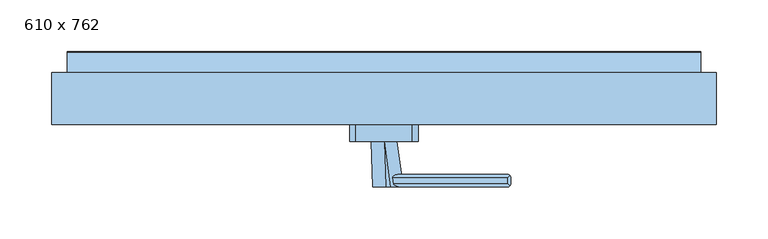
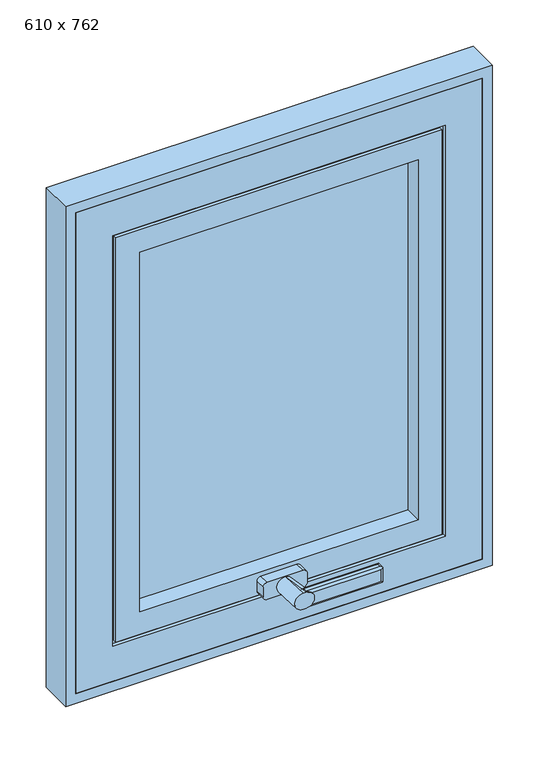
"""IFC4 building model written with IfcOpenShell, lengths in millimetres: window geometry, 610 x 762."""

from ifc_helpers import new_model, si_unit, point, frame, frame_2d, origin, place, context, project, spatial, polyline, circle_curve, ellipse_curve, trimmed, segment, composite_curve, outline, extrude, faceted_brep, source, transform, mapped, element, save
from ifc_brep_helpers import plane_surface, cylinder_surface, extruded_surface, advanced_brep


def window_610_x_762_22856471(model_context):
    return source(origin(), model_context, "Body", "SolidModel", [
        advanced_brep(
        [(6.2046905, -15.7, 888.0038591), (1.7209614, -15.7, 888.0038591), (1.7209614, -15.7, 863.0038591), (6.2046905, -15.7, 863.0038591), (0.0, 28.3, 888.0038591), (0.0, 28.3, 863.0038591)],
        [
            (0, 1),
            (1, 2, circle_curve(frame((1.7209614, -15.7, 875.5038591), z_axis=(0.0, -1.0, 0.0), x_axis=(1.0, 0.0, 0.0)), 12.5)),
            (2, 3),
            (3, 0, circle_curve(frame((6.2046905, -15.7, 875.5038591), z_axis=(0.0, -1.0, 0.0), x_axis=(1.0, 0.0, 0.0)), 12.5)),
            (4, 5, circle_curve(frame((0.0, 28.3, 875.5038591), z_axis=(0.0, 1.0, 0.0), x_axis=(1.0, 0.0, 0.0)), 12.5)),
            (5, 4, circle_curve(frame((0.0, 28.3, 875.5038591), z_axis=(0.0, 1.0, 0.0), x_axis=(1.0, 0.0, 0.0)), 12.5)),
            (5, 2),
            (1, 4),
            (0, 4),
            (5, 3),
        ],
        [
            plane_surface(frame((3.9628259, -15.7, 875.5038591), z_axis=(0.0, -1.0, 0.0), x_axis=(-1.0, 0.0, 0.0))),
            plane_surface(frame((0.0, 28.3, 875.5038591), z_axis=(0.0, 1.0, 0.0), x_axis=(-1.0, 0.0, 0.0))),
            extruded_surface(trimmed(circle_curve(frame((0.0, 28.3, 875.5038591), z_axis=(0.0, -1.0, 0.0), x_axis=(1.0, 0.0, 0.0)), 12.5), [point((0.0, 28.3, 888.0038591))], [point((0.0, 28.3, 863.0038591))], True, "CARTESIAN"), (1.7209614, -44.0, 0.0), 44.03364291244014),
            plane_surface(frame((0.0, 28.3, 888.0038591), z_axis=(0.0, 0.0, 1.0), x_axis=(-1.0, 0.0, 0.0))),
            plane_surface(frame((0.0, 28.3, 863.0038591), z_axis=(0.0, 0.0, -1.0), x_axis=(1.0, 0.0, 0.0))),
            extruded_surface(trimmed(circle_curve(frame((0.0, 28.3, 875.5038591), z_axis=(0.0, -1.0, 0.0), x_axis=(1.0, 0.0, 0.0)), 12.5), [point((0.0, 28.3, 863.0038591))], [point((0.0, 28.3, 888.0038591))], True, "CARTESIAN"), (6.2046905, -44.0, 0.0), 44.43532585905937),
        ],
        [
            (0, [[1, 2, 3, 4]]),
            (1, [[5, 6]]),
            (2, [[-6, 7, -2, 8]]),
            (3, [[-1, 9, -8]]),
            (4, [[-3, -7, 10]]),
            (5, [[-5, -9, -4, -10]]),
        ],
    ),
        advanced_brep(
        [(122.0, -12.7, 866.0038591), (122.0, -6.7, 866.0038591), (122.0, -6.7, 885.0038591), (122.0, -12.7, 885.0038591), (4.7741708, -15.7, 866.0038591), (4.7741708, -12.7, 863.0038591), (110.9250215, -12.7, 863.0038591), (119.0, -12.7, 863.0038591), (121.1213203, -14.8213203, 863.8825388), (119.0, -15.7, 866.0038591), (113.6581962, -15.7, 866.0038591), (4.7741708, -6.7, 863.0038591), (4.7741708, -3.7, 866.0038591), (113.6581962, -3.7, 866.0038591), (119.0, -3.7, 866.0038591), (121.1213203, -4.5786797, 863.8825388), (119.0, -6.7, 863.0038591), (110.9250215, -6.7, 863.0038591), (4.7741708, -3.7, 885.0038591), (113.6581962, -3.7, 885.0038591), (119.0, -3.7, 885.0038591), (4.7741708, -6.7, 888.0038591), (110.9250215, -6.7, 888.0038591), (119.0, -6.7, 888.0038591), (121.1213203, -4.5786797, 887.1251795), (4.7741708, -12.7, 888.0038591), (4.7741708, -15.7, 885.0038591), (113.6581962, -15.7, 885.0038591), (119.0, -15.7, 885.0038591), (121.1213203, -14.8213203, 887.1251795), (119.0, -12.7, 888.0038591), (110.9250215, -12.7, 888.0038591)],
        [
            (0, 1),
            (1, 2),
            (2, 3),
            (3, 0),
            (4, 5, circle_curve(frame((4.7741708, -12.7, 866.0038591), z_axis=(1.0, 0.0, 0.0), x_axis=(0.0, 0.0, 1.0)), 3.0)),
            (5, 6),
            (6, 7),
            (7, 8, ellipse_curve(frame((119.0, -12.7, 866.0038591), z_axis=(-0.7071067811865427, -0.7071067811865525, 0.0), x_axis=(0.7071067811865522, -0.7071067811865428, 0.0)), 4.2426407, 3.0)),
            (8, 9, ellipse_curve(frame((119.0, -12.7, 866.0038591), z_axis=(-0.70710678118655, 0.0, -0.7071067811865449), x_axis=(0.7071067811865451, 0.0, -0.7071067811865498)), 4.2426407, 3.0)),
            (9, 10),
            (10, 4),
            (11, 12, circle_curve(frame((4.7741708, -6.7, 866.0038591), z_axis=(1.0, 0.0, 0.0), x_axis=(0.0, 0.0, 1.0)), 3.0)),
            (12, 13),
            (13, 14),
            (14, 15, ellipse_curve(frame((119.0, -6.7, 866.0038591), z_axis=(-0.70710678118655, 0.0, -0.7071067811865449), x_axis=(0.7071067811865451, 0.0, -0.7071067811865498)), 4.2426407, 3.0)),
            (15, 16, ellipse_curve(frame((119.0, -6.7, 866.0038591), z_axis=(-0.7071067811865523, 0.7071067811865426, 0.0), x_axis=(0.7071067811865428, 0.7071067811865522, 0.0)), 4.2426407, 3.0)),
            (16, 17),
            (17, 11),
            (12, 18),
            (18, 19),
            (19, 20),
            (20, 14),
            (18, 21, circle_curve(frame((4.7741708, -6.7, 885.0038591), z_axis=(1.0, 0.0, 0.0), x_axis=(0.0, 0.0, 1.0)), 3.0)),
            (21, 22),
            (22, 23),
            (23, 24, ellipse_curve(frame((119.0, -6.7, 885.0038591), z_axis=(-0.7071067811865523, 0.7071067811865426, 0.0), x_axis=(0.7071067811865428, 0.7071067811865522, 0.0)), 4.2426407, 3.0)),
            (24, 20, ellipse_curve(frame((119.0, -6.7, 885.0038591), z_axis=(-0.7071067811865449, 0.0, 0.70710678118655), x_axis=(0.7071067811865501, 0.0, 0.7071067811865448)), 4.2426407, 3.0)),
            (25, 26, circle_curve(frame((4.7741708, -12.7, 885.0038591), z_axis=(1.0, 0.0, 0.0), x_axis=(0.0, 0.0, 1.0)), 3.0)),
            (26, 27),
            (27, 28),
            (28, 29, ellipse_curve(frame((119.0, -12.7, 885.0038591), z_axis=(-0.7071067811865449, 0.0, 0.70710678118655), x_axis=(0.7071067811865501, 0.0, 0.7071067811865448)), 4.2426407, 3.0)),
            (29, 30, ellipse_curve(frame((119.0, -12.7, 885.0038591), z_axis=(-0.7071067811865427, -0.7071067811865525, 0.0), x_axis=(0.7071067811865522, -0.7071067811865428, 0.0)), 4.2426407, 3.0)),
            (30, 31),
            (31, 25),
            (23, 30),
            (29, 3, ellipse_curve(frame((119.0, -12.7, 885.0038591), z_axis=(0.0, 0.7071067811865499, 0.707106781186545), x_axis=(0.0, 0.7071067811865451, -0.7071067811865498)), 4.2426407, 3.0)),
            (2, 24, ellipse_curve(frame((119.0, -6.7, 885.0038591), z_axis=(0.0, -0.7071067811865451, 0.7071067811865499), x_axis=(0.0, 0.70710678118655, 0.7071067811865451)), 4.2426407, 3.0)),
            (7, 16),
            (15, 1, ellipse_curve(frame((119.0, -6.7, 866.0038591), z_axis=(0.0, -0.7071067811865499, -0.707106781186545), x_axis=(0.0, 0.7071067811865451, -0.7071067811865498)), 4.2426407, 3.0)),
            (0, 8, ellipse_curve(frame((119.0, -12.7, 866.0038591), z_axis=(0.0, 0.7071067811865451, -0.7071067811865499), x_axis=(0.0, 0.70710678118655, 0.7071067811865451)), 4.2426407, 3.0)),
            (28, 9),
            (25, 21),
            (11, 5),
            (4, 26),
        ],
        [
            plane_surface(frame((122.0, -15.7, 863.0038591), z_axis=(1.0, 0.0, 0.0), x_axis=(0.0, 0.0, -1.0))),
            cylinder_surface(frame((4.7741708, -12.7, 866.0038591), z_axis=(1.0, 0.0, 0.0), x_axis=(0.0, 0.0, 1.0)), 3.0),
            cylinder_surface(frame((4.7741708, -6.7, 866.0038591), z_axis=(1.0, 0.0, 0.0), x_axis=(0.0, 0.0, 1.0)), 3.0),
            plane_surface(frame((122.0, -3.7, 866.0038591), z_axis=(0.0, 1.0, 0.0), x_axis=(-1.0, 0.0, 0.0))),
            cylinder_surface(frame((4.7741708, -6.7, 885.0038591), z_axis=(1.0, 0.0, 0.0), x_axis=(0.0, 0.0, 1.0)), 3.0),
            cylinder_surface(frame((4.7741708, -12.7, 885.0038591), z_axis=(1.0, 0.0, 0.0), x_axis=(0.0, 0.0, 1.0)), 3.0),
            cylinder_surface(frame((119.0, -3.7, 885.0038591), z_axis=(0.0, 1.0, 0.0), x_axis=(0.0, 0.0, 1.0)), 3.0),
            cylinder_surface(frame((119.0, -3.7, 866.0038591), z_axis=(0.0, 1.0, 0.0), x_axis=(0.0, 0.0, 1.0)), 3.0),
            cylinder_surface(frame((119.0, -6.7, 862.0038591), z_axis=(0.0, 0.0, -1.0), x_axis=(-1.0, 0.0, 0.0)), 3.0),
            cylinder_surface(frame((119.0, -12.7, 862.0038591), z_axis=(0.0, 0.0, -1.0), x_axis=(-1.0, 0.0, 0.0)), 3.0),
            plane_surface(frame((4.7741708, -15.7, 863.0038591), z_axis=(-1.0, 0.0, 0.0), x_axis=(0.0, 0.0, 1.0))),
            plane_surface(frame((122.0, -15.7, 885.0038591), z_axis=(0.0, -1.0, 0.0), x_axis=(-1.0, 0.0, 0.0))),
            plane_surface(frame((122.0, -12.7, 863.0038591), z_axis=(0.0, 0.0, -1.0), x_axis=(-1.0, 0.0, 0.0))),
            plane_surface(frame((122.0, -6.7, 888.0038591), z_axis=(0.0, 0.0, 1.0), x_axis=(-1.0, 0.0, 0.0))),
        ],
        [
            (0, [[1, 2, 3, 4]]),
            (1, [[5, 6, 7, 8, 9, 10, 11]]),
            (2, [[12, 13, 14, 15, 16, 17, 18]]),
            (3, [[19, 20, 21, 22, -14, -13]]),
            (4, [[23, 24, 25, 26, 27, -21, -20]]),
            (5, [[28, 29, 30, 31, 32, 33, 34]]),
            (6, [[35, -32, 36, -3, 37, -26]]),
            (7, [[38, -16, 39, -1, 40, -8]]),
            (8, [[-2, -39, -15, -22, -27, -37]]),
            (9, [[-4, -36, -31, 41, -9, -40]]),
            (10, [[-28, 42, -23, -19, -12, 43, -5, 44]]),
            (11, [[-44, -11, -10, -41, -30, -29]]),
            (12, [[-43, -18, -17, -38, -7, -6]]),
            (13, [[-42, -34, -33, -35, -25, -24]]),
        ],
    ),
        extrude(outline(composite_curve([segment(polyline([(883.0038591, -33.0), (868.0038591, -33.0)]), True, "CONTINUOUS"), segment(trimmed(circle_curve(frame_2d((868.0038591, -27.0)), 6.0), [point((868.0038591, -33.0))], [point((862.0038591, -27.0))], False, "CARTESIAN"), True, "CONTINUOUS"), segment(polyline([(862.0038591, -27.0), (862.0038591, 27.0)]), True, "CONTINUOUS"), segment(trimmed(circle_curve(frame_2d((868.0038591, 27.0)), 6.0), [point((862.0038591, 27.0))], [point((868.0038591, 33.0))], False, "CARTESIAN"), True, "CONTINUOUS"), segment(polyline([(868.0038591, 33.0), (883.0038591, 33.0)]), True, "CONTINUOUS"), segment(trimmed(circle_curve(frame_2d((883.0038591, 27.0)), 6.0), [point((883.0038591, 33.0))], [point((889.0038591, 27.0))], False, "CARTESIAN"), True, "CONTINUOUS"), segment(polyline([(889.0038591, 27.0), (889.0038591, -27.0)]), True, "CONTINUOUS"), segment(trimmed(circle_curve(frame_2d((883.0038591, -27.0)), 6.0), [point((889.0038591, -27.0))], [point((883.0038591, -33.0))], False, "CARTESIAN"), True, "CONTINUOUS")], self_intersect=False)), frame((0.0, 28.3, 0.0), z_axis=(0.0, 1.0, 0.0), x_axis=(0.0, 0.0, 1.0)), (0.0, 0.0, 1.0), 16.0),
        extrude(outline(polyline([(785.0, -319.8), (785.0, 319.8), (1577.0, 319.8), (1577.0, -319.8), (785.0, -319.8)]), holes=[polyline([(1562.0, -304.8), (1562.0, 304.8), (800.0, 304.8), (800.0, -304.8), (1562.0, -304.8)])]), frame((0.0, 44.3, 0.0), z_axis=(0.0, 1.0, 0.0), x_axis=(0.0, 0.0, 1.0)), (0.0, 0.0, 1.0), 50.0),
        faceted_brep([(-304.8, 44.3, 1562.0), (-304.8, 94.3, 1562.0), (-304.8, 94.3, 800.0), (-304.8, 44.3, 800.0), (-271.3, 94.3, 1528.5), (-271.3, 49.5, 1528.5), (-271.3, 49.5, 833.5), (-271.3, 94.3, 833.5), (-249.3, 49.5, 1506.5), (-249.3, 44.3, 1506.5), (-249.3, 44.3, 855.5), (-249.3, 49.5, 855.5), (304.8, 94.3, 800.0), (304.8, 44.3, 800.0), (271.3, 49.5, 833.5), (271.3, 94.3, 833.5), (249.3, 44.3, 855.5), (249.3, 49.5, 855.5), (304.8, 94.3, 1562.0), (304.8, 44.3, 1562.0), (271.3, 49.5, 1528.5), (271.3, 94.3, 1528.5), (249.3, 44.3, 1506.5), (249.3, 49.5, 1506.5)], [[[0, 1, 2, 3]], [[4, 5, 6, 7]], [[8, 9, 10, 11]], [[3, 2, 12, 13]], [[7, 6, 14, 15]], [[11, 10, 16, 17]], [[13, 12, 18, 19]], [[15, 14, 20, 21]], [[17, 16, 22, 23]], [[19, 18, 1, 0]], [[1, 18, 12, 2], [7, 15, 21, 4]], [[21, 20, 5, 4]], [[5, 20, 14, 6], [11, 17, 23, 8]], [[23, 22, 9, 8]], [[3, 13, 19, 0], [9, 22, 16, 10]]]),
        extrude(outline(polyline([(-220.8, 70.8), (-220.8, 94.8), (220.8, 94.8), (220.8, 70.8), (-220.8, 70.8)])), frame((0.0, 0.0, 884.0), z_axis=(0.0, 0.0, 1.0), x_axis=(1.0, 0.0, 0.0)), (0.0, 0.0, 1.0), 594.0),
        faceted_brep([(277.3, 103.3, 1534.5), (277.3, 94.3, 1534.5), (277.3, 94.3, 827.5), (277.3, 103.3, 827.5), (204.8, 94.8, 1462.0), (204.8, 103.3, 1462.0), (204.8, 103.3, 900.0), (204.8, 94.8, 900.0), (220.8, 70.8, 1478.0), (220.8, 94.8, 1478.0), (220.8, 94.8, 884.0), (220.8, 70.8, 884.0), (208.8, 44.3, 1466.0), (208.8, 70.8, 1466.0), (208.8, 70.8, 896.0), (208.8, 44.3, 896.0), (244.3, 49.5, 1501.5), (244.3, 44.3, 1501.5), (244.3, 44.3, 860.5), (244.3, 49.5, 860.5), (259.9392195, 94.3, 1517.1392195), (259.9392195, 49.5, 1517.1392195), (259.9392195, 49.5, 844.8607805), (259.9392195, 94.3, 844.8607805), (-277.3, 94.3, 827.5), (-277.3, 103.3, 827.5), (-204.8, 103.3, 900.0), (-204.8, 94.8, 900.0), (-220.8, 94.8, 884.0), (-220.8, 70.8, 884.0), (-208.8, 70.8, 896.0), (-208.8, 44.3, 896.0), (-244.3, 44.3, 860.5), (-244.3, 49.5, 860.5), (-259.9392195, 49.5, 844.8607805), (-259.9392195, 94.3, 844.8607805), (-277.3, 94.3, 1534.5), (-277.3, 103.3, 1534.5), (-204.8, 103.3, 1462.0), (-204.8, 94.8, 1462.0), (-220.8, 94.8, 1478.0), (-220.8, 70.8, 1478.0), (-208.8, 70.8, 1466.0), (-208.8, 44.3, 1466.0), (-244.3, 44.3, 1501.5), (-244.3, 49.5, 1501.5), (-259.9392195, 49.5, 1517.1392195), (-259.9392195, 94.3, 1517.1392195)], [[[0, 1, 2, 3]], [[4, 5, 6, 7]], [[8, 9, 10, 11]], [[12, 13, 14, 15]], [[16, 17, 18, 19]], [[20, 21, 22, 23]], [[3, 2, 24, 25]], [[7, 6, 26, 27]], [[11, 10, 28, 29]], [[15, 14, 30, 31]], [[19, 18, 32, 33]], [[23, 22, 34, 35]], [[25, 24, 36, 37]], [[27, 26, 38, 39]], [[29, 28, 40, 41]], [[31, 30, 42, 43]], [[33, 32, 44, 45]], [[35, 34, 46, 47]], [[37, 36, 1, 0]], [[3, 25, 37, 0], [5, 38, 26, 6]], [[39, 38, 5, 4]], [[9, 40, 28, 10], [7, 27, 39, 4]], [[41, 40, 9, 8]], [[11, 29, 41, 8], [13, 42, 30, 14]], [[43, 42, 13, 12]], [[17, 44, 32, 18], [15, 31, 43, 12]], [[45, 44, 17, 16]], [[21, 46, 34, 22], [19, 33, 45, 16]], [[47, 46, 21, 20]], [[1, 36, 24, 2], [23, 35, 47, 20]]]),
        extrude(outline(polyline([(94.3, 1547.0), (94.3, 1562.0421053), (113.5, 1558.0), (114.5, 1552.0), (113.0, 1552.0), (111.751709, 1556.3242199), (98.5146457, 1559.11097), (95.9649679, 1547.0), (94.3, 1547.0)])), frame((-304.8, 0.0, 0.0), z_axis=(1.0, 0.0, 0.0), x_axis=(0.0, 1.0, 0.0)), (0.0, 0.0, 1.0), 609.6),
    ])


if __name__ == "__main__":
    model = new_model("IFC4")
    model_context = context("Model", 3, world=origin())
    ifc_project = project(units=[si_unit("LENGTHUNIT", "METRE", prefix="MILLI")], contexts=[model_context])
    site = spatial("IfcSite", under=ifc_project)
    building = spatial("IfcBuilding", under=site)
    placement = place(None, origin())
    window_610_x_762_shape = window_610_x_762_22856471(model_context)
    element("IfcWindow", 1, ObjectType="610 x 762", at=placement, inside=building, context=model_context, shape_type="MappedRepresentation", body=[
        mapped(window_610_x_762_shape, transform((0.0, 0.0, 0.0), x_axis=(1.0, 0.0, 0.0), y_axis=(0.0, 1.0, 0.0), z_axis=(0.0, 0.0, 1.0))),
    ])
    save(model, "model.ifc")

# Revit data of these elements
# Type "610 x 762"
#   Type Mark = "18"
#   Water resistance = "up to Class E1050, PN-EN 12208:2001"
#   URL = "https://aluprof.com/en/architects/offer/window-and-door-systems/mb-59s-casement-mb-59s-casement-hi"
#   Type IFC Predefined Type = "NOTDEFINED"
#   Resistance to wind load = "up to Class C5, PN-EN 12210:2016"
#   Operation = "SingleTopHungCasement"
#   Opening type = "Top-hung casement opening outwards"
#   Model = "MB-59S Casement"
#   ManufacturerSustainabilityPolicyURL = "https://aluprof.eu/en/company/sustainable-development"
#   Manufacturer = "ALUPROF SA"
#   Keynote = "08511300"
#   IfcExportType = "NOTDEFINED"
#   IfcExportAs = "IfcWindowType"
#   Hardware [instance default] = ""
#   Handle type [instance default] = ""
#   Glazing construction = "4/16/4"
#   Export Type to IFC As = "IfcWindowType"
#   Description = "Single top-hung casement opening outwards"
#   Content of the recyclate in the material = "69.2%"
#   COBie.Type.Name = "MB-59S Casement"
#   COBie.Type.Manufacturer = "ALUPROF SA\r\nALUPROF S.A.\r\nALUPROF S.A."
#   Assembly Code = "B2020110"
#   Analytic Construction = "<None>"
#   Air permeability = "up to Class 4, PN-EN 12207:2001"
#   Thermal insulation = 0.299387 BTU/(h·ft²·°F)
#   Sash thickness = 0' - 2.32283"
#   Rough Width = 2' - 1.1811"
#   Rough Height = 2' - 7.1811"
#   Reference line height [instance default] = 0' - 0"
#   Opening angle [instance default] = 0.00°
#   Mounting space = 0' - 0.59055"
#   Height = 2' - 6"
#   Glazing area = 2.82349 SF
#   Frame thickness = 0' - 1.9685"
#   Exterior wall face offset = 0' - 0.7874"
#   Sill Height = 2' - 7.49606"
#   Width = 2' - 0"
#   Warm installation [instance default] = yes
#   Thermal variant HI = no
#   Schedule No. [instance default] = 1
#   IsWindowOpen [instance default] = no
#   IsExternal = yes
#   Define Thermal Properties by = 1
#   COBie.Type = yes
#   COBie = yes
#   Wall Closure = (empty or 0)
